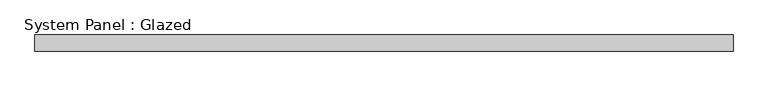
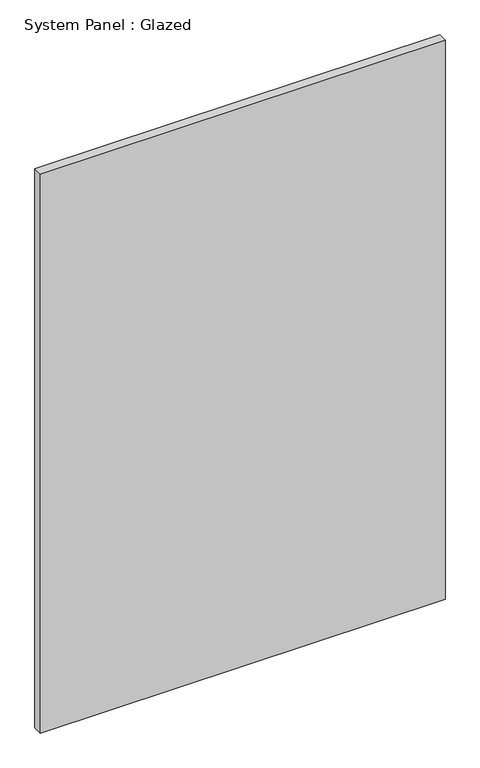
"""IFC4 building model written with IfcOpenShell, lengths in millimetres: plate geometry, System Panel : Glazed."""

from ifc_helpers import new_model, si_unit, origin, origin_with_axes, place, context, project, spatial, polyline, outline, extrude, source, transform, mapped, element, save


def system_panel_glazed_74a1dbaf(model_context):
    return source(origin(), model_context, "Body", "SweptSolid", [
        extrude(outline(polyline([(528.0, 24.5), (-528.0, 24.5), (-528.0, 49.5), (528.0, 49.5), (528.0, 24.5)])), origin_with_axes(), (0.0, 0.0, 1.0), 1541.6),
    ])


if __name__ == "__main__":
    model = new_model("IFC4")
    model_context = context("Model", 3, world=origin())
    ifc_project = project(units=[si_unit("LENGTHUNIT", "METRE", prefix="MILLI")], contexts=[model_context])
    site = spatial("IfcSite", under=ifc_project)
    building = spatial("IfcBuilding", under=site)
    placement = place(None, origin())
    system_panel_glazed_shape = system_panel_glazed_74a1dbaf(model_context)
    element("IfcPlate", 1, ObjectType="System Panel : Glazed", at=placement, inside=building, context=model_context, shape_type="MappedRepresentation", body=[
        mapped(system_panel_glazed_shape, transform((0.0, 0.0, 0.0), x_axis=(1.0, 0.0, 0.0), y_axis=(0.0, 1.0, 0.0), z_axis=(0.0, 0.0, 1.0))),
    ])
    save(model, "model.ifc")

# Revit data of these elements
# Type "System Panel : Glazed"
#   Construction Type Id = "GSP4R"
#   Analytic Construction = "1/8 in Pilkington single glazing"
#   Visual Light Transmittance = 0.9
#   Solar Heat Gain Coefficient = 0.86
#   Heat Transfer Coefficient (U) = 6.7069 W/(m²·K)
#   Define Thermal Properties by = 1
# Element 1 (IfcPlate, "System Panel : Glazed")
#   Materials on its faces: "Glass"
# Materials
#   "Glass": class "Glass", colour RGB 0 128 192, transparency 0.9, Description = "Soda Lime Glass", Cost = 0
